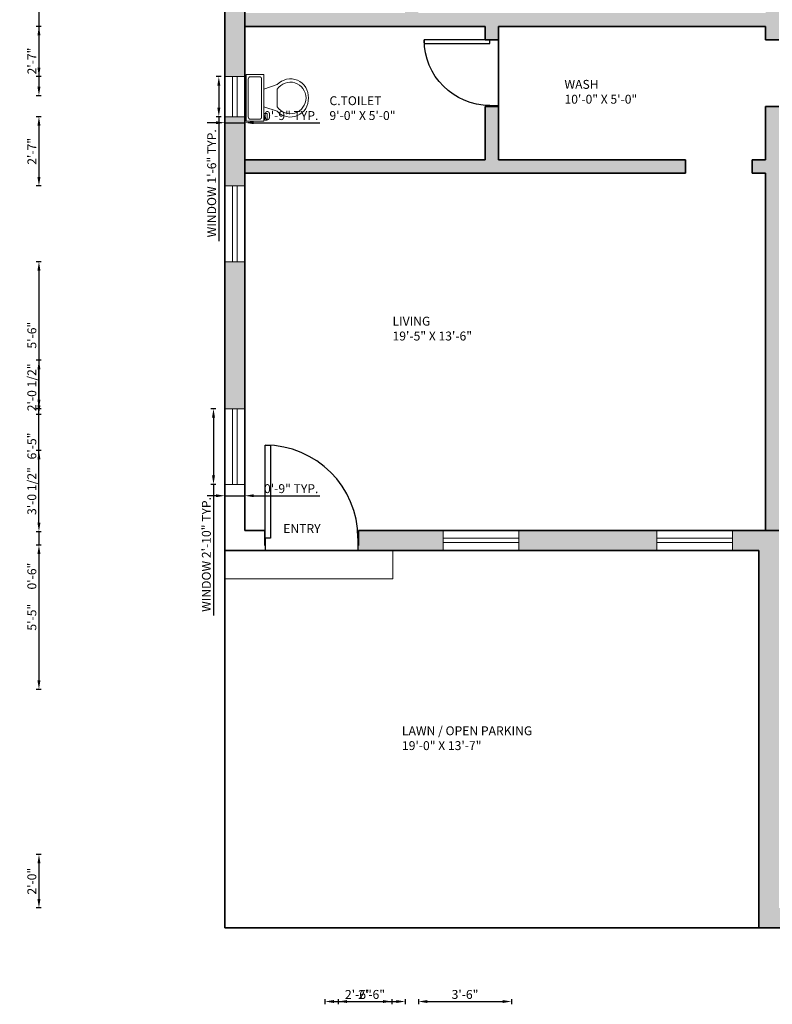
# Model space of a CAD drawing. Units: inches. Extents: x -91 to 518, y -600 to 105.
# Tile 1 of 4: x -91 to 248, y -598 to -155. Entities that reach past the tile are written whole.
import ezdxf

# ---------------------------------------------------------------- set-up
doc = ezdxf.new("R2010")
doc.units = ezdxf.units.IN
for name, color, linetype, lineweight in [('A-ANNO-DIMS', 2, 'Continuous', 18), ('A-ANNO-TEXT', 7, 'Continuous', 18), ('A-AREA-IDEN', 7, 'Continuous', 18), ('A-DOOR', 4, 'Continuous', 25), ('A-FLOR-FIXT', 9, 'Continuous', 18), ('A-FLOR-STRS', 7, 'Continuous', 18), ('A-GLAZ', 6, 'Continuous', 18), ('A-WALL', 7, 'Continuous', 35), ('A-WALL-PATT', 251, 'Continuous', 13)]:
    doc.layers.add(name, color=color, linetype=linetype, lineweight=lineweight)
doc.styles.get("Standard").update_dxf_attribs({"font": 'arial.ttf'})
doc.dimstyles.new('ISO-25', dxfattribs={"dimtxt": 4, "dimasz": 4, "dimexe": 1.25, "dimexo": 0.625, "dimtad": 1, "dimlunit": 3, "dimtxsty": 'Standard', "dimcen": 2.5, "dimadec": 0, "dimazin": 0, "dimtfac": 1, "dimtmove": 0, "dimatfit": 3, "dimfxl": 1, "dimfxlon": 1, "dimarcsym": 0})

# ---------------------------------------------------------------- blocks, each defined once
blk = doc.blocks.new('*U4')
for p, q in [((9.5, -6), (9.5, -2)), ((-10, -8.5), (-8, -8.5)), ((-10, -9.5), (-10, -8.5)), ((-8, -8.5), (-8, -8)), ((-7, -8), (-7, -9.5)), ((-4, -8), (-6, -14)), ((4, -8), (6, -14)), ((-7, -9.5), (-10, -9.5)), ((4, -14), (-4, -14))]:
    blk.add_line(p, q)
blk.add_lwpolyline([(10.5, -8), (10.5, 0), (-10.5, 0), (-10.5, -8)], close=True)
for points in [[(-9.5, -2), (-9.5, -6)], [(8.5, -1), (-8.5, -1)], [(-8.5, -7), (8.5, -7)]]:
    blk.add_lwpolyline(points)
for centre, radius, start, end in [((-8.625, -1.875), 0.8839, 81.8699, 188.1301), ((8.625, -1.875), 0.8839, 351.8699, 98.1301), ((-8.625, -6.125), 0.8839, 171.869898, 278.1301), ((8.625, -6.125), 0.8839, 261.8699, 8.1301), ((-0.4772, -19.9188), 8.0953, 133.01722, 273.38), ((0.0374, -19.8731), 7.127, 124.50543, 269.7), ((-0.0373, -19.8731), 7.127, 270.3, 55.4946), ((0.4773, -19.9188), 8.0953, 266.62, 46.9828)]:
    blk.add_arc(centre, radius, start, end)
blk = doc.blocks.new('*U2')
for p, q in [((0, 0), (0, -100)), ((750, 0), (750, -100))]:
    blk.add_line(p, q)
blk.add_lwpolyline([(0, 0), (0, 750), (43.75, 750), (43.75, 0)], close=True)
blk.add_arc((0, 0), 750, 0, 90)
blk = doc.blocks.new('WIN-34IN')
for p, q in [((0, 5.5), (34, 5.5)), ((0, 3.5), (34, 3.5))]:
    blk.add_line(p, q)
blk.add_lwpolyline([(0, 9), (34, 9), (34, 0), (0, 0)], close=True)
blk = doc.blocks.new('WIN-18IN')
for p, q in [((0, 5.5), (18, 5.5)), ((0, 3.5), (18, 3.5))]:
    blk.add_line(p, q)
blk.add_lwpolyline([(0, 9), (18, 9), (18, 0), (0, 0)], close=True)
blk = doc.blocks.new('*D18')
at = {"layer": 'A-ANNO-DIMS', "color": 0, "lineweight": -2, "transparency": 16777216}
for p, q in [((-2.56, -330.05), (-4.81, -330.05)), ((-3.56, -334.05), (-3.56, -360.05)), ((-2.56, -364.05), (-4.81, -364.05)), ((-3.56, -364.05), (-3.56, -423.02))]:
    blk.add_line(p, q, dxfattribs=at)
at = {"layer": 'A-ANNO-DIMS', "color": 0, "transparency": 16777216}
for points in [[(-4.22, -334.05), (-2.89, -334.05), (-3.56, -330.05)], [(-4.22, -360.05), (-2.89, -360.05), (-3.56, -364.05)]]:
    blk.add_solid(points, dxfattribs=at)
at = {"layer": 'Defpoints', "color": 0, "transparency": 16777216}
for p in [(1.54, -330.05), (-3.56, -364.05), (1.54, -364.05)]:
    blk.add_point(p, dxfattribs=at)
at = {"layer": 'A-ANNO-DIMS', "color": 0, "transparency": 16777216, "insert": (-6.25, -395.53), "char_height": 4, "attachment_point": 5, "rotation": 90}
blk.add_mtext('WINDOW 2\'-10" TYP.', dxfattribs=at)
blk = doc.blocks.new('*D19')
at = {"layer": 'A-ANNO-DIMS', "color": 0, "lineweight": -2, "transparency": 16777216}
for p, q in [((-2.46, -369.15), (-6.46, -369.15)), ((1.54, -368.15), (1.54, -370.4)), ((1.54, -369.15), (10.54, -369.15)), ((10.54, -368.15), (10.54, -370.4)), ((14.54, -369.15), (44.18, -369.15))]:
    blk.add_line(p, q, dxfattribs=at)
at = {"layer": 'A-ANNO-DIMS', "color": 0, "transparency": 16777216}
for points in [[(-2.46, -368.48), (-2.46, -369.81), (1.54, -369.15)], [(14.54, -368.48), (14.54, -369.81), (10.54, -369.15)]]:
    blk.add_solid(points, dxfattribs=at)
at = {"layer": 'Defpoints', "color": 0, "transparency": 16777216}
for p in [(1.54, -364.05), (10.54, -364.05), (10.54, -369.15)]:
    blk.add_point(p, dxfattribs=at)
at = {"layer": 'A-ANNO-DIMS', "color": 0, "transparency": 16777216, "insert": (31.36, -366.48), "char_height": 4, "attachment_point": 5}
blk.add_mtext('0\'-9" TYP.', dxfattribs=at)
blk = doc.blocks.new('*D20')
at = {"layer": 'A-ANNO-DIMS', "color": 0, "lineweight": -2, "transparency": 16777216}
for p, q in [((-0.16, -180.88), (-2.41, -180.88)), ((-1.16, -184.88), (-1.16, -194.88)), ((-0.16, -198.88), (-2.41, -198.88)), ((-1.16, -198.88), (-1.16, -254.74))]:
    blk.add_line(p, q, dxfattribs=at)
at = {"layer": 'A-ANNO-DIMS', "color": 0, "transparency": 16777216}
for points in [[(-1.82, -184.88), (-0.49, -184.88), (-1.16, -180.88)], [(-1.82, -194.88), (-0.49, -194.88), (-1.16, -198.88)]]:
    blk.add_solid(points, dxfattribs=at)
at = {"layer": 'Defpoints', "color": 0, "transparency": 16777216}
for p in [(1.54, -180.88), (-1.16, -198.88), (1.54, -198.88)]:
    blk.add_point(p, dxfattribs=at)
at = {"layer": 'A-ANNO-DIMS', "color": 0, "transparency": 16777216, "insert": (-3.85, -228.81), "char_height": 4, "attachment_point": 5, "rotation": 90}
blk.add_mtext('WINDOW 1\'-6" TYP.', dxfattribs=at)
blk = doc.blocks.new('*D21')
at = {"layer": 'A-ANNO-DIMS', "color": 0, "lineweight": -2, "transparency": 16777216}
for p, q in [((-2.46, -201.58), (-6.46, -201.58)), ((1.54, -200.58), (1.54, -202.83)), ((1.54, -201.58), (10.54, -201.58)), ((10.54, -200.58), (10.54, -202.83)), ((14.54, -201.58), (44.18, -201.58))]:
    blk.add_line(p, q, dxfattribs=at)
at = {"layer": 'A-ANNO-DIMS', "color": 0, "transparency": 16777216}
for points in [[(-2.46, -200.91), (-2.46, -202.24), (1.54, -201.58)], [(14.54, -200.91), (14.54, -202.24), (10.54, -201.58)]]:
    blk.add_solid(points, dxfattribs=at)
at = {"layer": 'Defpoints', "color": 0, "transparency": 16777216}
for p in [(1.54, -198.88), (10.54, -198.88), (10.54, -201.58)]:
    blk.add_point(p, dxfattribs=at)
at = {"layer": 'A-ANNO-DIMS', "color": 0, "transparency": 16777216, "insert": (31.36, -198.91), "char_height": 4, "attachment_point": 5}
blk.add_mtext('0\'-9" TYP.', dxfattribs=at)
blk = doc.blocks.new('*D32')
at = {"layer": 'A-ANNO-DIMS', "color": 0, "lineweight": -2, "transparency": 16777216}
for p, q in [((19.54, 95.59), (19.54, 97.84)), ((61.54, 95.59), (61.54, 97.84)), ((23.54, 96.59), (57.54, 96.59))]:
    blk.add_line(p, q, dxfattribs=at)
at = {"layer": 'A-ANNO-DIMS', "color": 0, "transparency": 16777216}
for points in [[(23.54, 97.25), (23.54, 95.92), (19.54, 96.59)], [(57.54, 97.25), (57.54, 95.92), (61.54, 96.59)]]:
    blk.add_solid(points, dxfattribs=at)
at = {"layer": 'Defpoints', "color": 0, "transparency": 16777216}
for p in [(61.54, 96.59), (19.54, -384.72), (61.54, -384.72)]:
    blk.add_point(p, dxfattribs=at)
at = {"layer": 'A-ANNO-DIMS', "color": 0, "transparency": 16777216, "insert": (40.54, 99.26), "char_height": 4, "attachment_point": 5}
blk.add_mtext('3\'-6"', dxfattribs=at)
blk = doc.blocks.new('*D34')
at = {"layer": 'A-ANNO-DIMS', "color": 0, "lineweight": -2, "transparency": 16777216}
for p, q in [((46.54, -595.36), (46.54, -597.61)), ((50.54, -596.36), (72.54, -596.36)), ((76.54, -595.36), (76.54, -597.61))]:
    blk.add_line(p, q, dxfattribs=at)
at = {"layer": 'A-ANNO-DIMS', "color": 0, "transparency": 16777216}
for points in [[(50.54, -595.69), (50.54, -597.02), (46.54, -596.36)], [(72.54, -595.69), (72.54, -597.02), (76.54, -596.36)]]:
    blk.add_solid(points, dxfattribs=at)
at = {"layer": 'Defpoints', "color": 0, "transparency": 16777216}
for p in [(46.54, -98.31), (76.54, -98.31), (76.54, -596.36)]:
    blk.add_point(p, dxfattribs=at)
at = {"layer": 'A-ANNO-DIMS', "color": 0, "transparency": 16777216, "insert": (61.54, -593.69), "char_height": 4, "attachment_point": 5}
blk.add_mtext('2\'-6"', dxfattribs=at)
blk = doc.blocks.new('*D35')
at = {"layer": 'A-ANNO-DIMS', "color": 0, "lineweight": -2, "transparency": 16777216}
for p, q in [((-81.99, -381.31), (-81.99, -377.31)), ((-80.99, -385.31), (-83.24, -385.31)), ((-81.99, -385.31), (-81.99, -391.31)), ((-80.99, -391.31), (-83.24, -391.31)), ((-81.99, -395.31), (-81.99, -411.19))]:
    blk.add_line(p, q, dxfattribs=at)
at = {"layer": 'A-ANNO-DIMS', "color": 0, "transparency": 16777216}
for points in [[(-82.66, -381.31), (-81.32, -381.31), (-81.99, -385.31)], [(-82.66, -395.31), (-81.32, -395.31), (-81.99, -391.31)]]:
    blk.add_solid(points, dxfattribs=at)
at = {"layer": 'Defpoints', "color": 0, "transparency": 16777216}
for p in [(310.54, -385.31), (-81.99, -391.31), (310.54, -391.31)]:
    blk.add_point(p, dxfattribs=at)
at = {"layer": 'A-ANNO-DIMS', "color": 0, "transparency": 16777216, "insert": (-84.66, -405.25), "char_height": 4, "attachment_point": 5, "rotation": 90}
blk.add_mtext('0\'-6"', dxfattribs=at)
blk = doc.blocks.new('*D36')
at = {"layer": 'A-ANNO-DIMS', "color": 0, "lineweight": -2, "transparency": 16777216}
for p, q in [((-80.99, -308.31), (-83.24, -308.31)), ((-81.99, -381.31), (-81.99, -312.31)), ((-80.99, -385.31), (-83.24, -385.31))]:
    blk.add_line(p, q, dxfattribs=at)
at = {"layer": 'A-ANNO-DIMS', "color": 0, "transparency": 16777216}
for points in [[(-82.66, -312.31), (-81.32, -312.31), (-81.99, -308.31)], [(-82.66, -381.31), (-81.32, -381.31), (-81.99, -385.31)]]:
    blk.add_solid(points, dxfattribs=at)
at = {"layer": 'Defpoints', "color": 0, "transparency": 16777216}
for p in [(-81.99, -308.31), (472.54, -308.31), (472.54, -385.31)]:
    blk.add_point(p, dxfattribs=at)
at = {"layer": 'A-ANNO-DIMS', "color": 0, "transparency": 16777216, "insert": (-84.66, -346.81), "char_height": 4, "attachment_point": 5, "rotation": 90}
blk.add_mtext('6\'-5"', dxfattribs=at)
blk = doc.blocks.new('*D37')
at = {"layer": 'A-ANNO-DIMS', "color": 0, "lineweight": -2, "transparency": 16777216}
for p, q in [((-80.99, -530.31), (-83.24, -530.31)), ((-81.99, -534.31), (-81.99, -550.31)), ((-80.99, -554.31), (-83.24, -554.31))]:
    blk.add_line(p, q, dxfattribs=at)
at = {"layer": 'A-ANNO-DIMS', "color": 0, "transparency": 16777216}
for points in [[(-82.66, -534.31), (-81.32, -534.31), (-81.99, -530.31)], [(-82.66, -550.31), (-81.32, -550.31), (-81.99, -554.31)]]:
    blk.add_solid(points, dxfattribs=at)
at = {"layer": 'Defpoints', "color": 0, "transparency": 16777216}
for p in [(375.09, -530.31), (-81.99, -554.31), (375.09, -554.31)]:
    blk.add_point(p, dxfattribs=at)
at = {"layer": 'A-ANNO-DIMS', "color": 0, "transparency": 16777216, "insert": (-84.66, -542.31), "char_height": 4, "attachment_point": 5, "rotation": 90}
blk.add_mtext('2\'-0"', dxfattribs=at)
blk = doc.blocks.new('*D41')
at = {"layer": 'A-ANNO-DIMS', "color": 0, "lineweight": -2, "transparency": 16777216}
for p, q in [((-80.99, 12.69), (-83.24, 12.69)), ((-81.99, 8.69), (-81.99, -176.88)), ((-80.99, -180.88), (-83.24, -180.88))]:
    blk.add_line(p, q, dxfattribs=at)
at = {"layer": 'A-ANNO-DIMS', "color": 0, "transparency": 16777216}
for points in [[(-82.66, 8.69), (-81.32, 8.69), (-81.99, 12.69)], [(-82.66, -176.88), (-81.32, -176.88), (-81.99, -180.88)]]:
    blk.add_solid(points, dxfattribs=at)
at = {"layer": 'Defpoints', "color": 0, "transparency": 16777216}
for p in [(1.54, 12.69), (-81.99, -180.88), (1.54, -180.88)]:
    blk.add_point(p, dxfattribs=at)
at = {"layer": 'A-ANNO-DIMS', "color": 0, "transparency": 16777216, "insert": (-84.68, -84.09), "char_height": 4, "attachment_point": 5, "rotation": 90}
blk.add_mtext('16\'-1 1/2"', dxfattribs=at)
blk = doc.blocks.new('*D42')
at = {"layer": 'A-ANNO-DIMS', "color": 0, "lineweight": -2, "transparency": 16777216}
for p, q in [((-80.99, -198.88), (-83.24, -198.88)), ((-81.99, -202.88), (-81.99, -226.01)), ((-80.99, -230.01), (-83.24, -230.01))]:
    blk.add_line(p, q, dxfattribs=at)
at = {"layer": 'A-ANNO-DIMS', "color": 0, "transparency": 16777216}
for points in [[(-82.66, -202.88), (-81.32, -202.88), (-81.99, -198.88)], [(-82.66, -226.01), (-81.32, -226.01), (-81.99, -230.01)]]:
    blk.add_solid(points, dxfattribs=at)
at = {"layer": 'Defpoints', "color": 0, "transparency": 16777216}
for p in [(1.54, -198.88), (-81.99, -230.01), (1.54, -230.01)]:
    blk.add_point(p, dxfattribs=at)
at = {"layer": 'A-ANNO-DIMS', "color": 0, "transparency": 16777216, "insert": (-84.62, -214.45), "char_height": 4, "attachment_point": 5, "rotation": 90}
blk.add_mtext('2\'-7"', dxfattribs=at)
blk = doc.blocks.new('*D43')
at = {"layer": 'A-ANNO-DIMS', "color": 0, "lineweight": -2, "transparency": 16777216}
for p, q in [((-80.99, -264.01), (-83.24, -264.01)), ((-81.99, -268.01), (-81.99, -326.05)), ((-80.99, -330.05), (-83.24, -330.05))]:
    blk.add_line(p, q, dxfattribs=at)
at = {"layer": 'A-ANNO-DIMS', "color": 0, "transparency": 16777216}
for points in [[(-82.66, -268.01), (-81.32, -268.01), (-81.99, -264.01)], [(-82.66, -326.05), (-81.32, -326.05), (-81.99, -330.05)]]:
    blk.add_solid(points, dxfattribs=at)
at = {"layer": 'Defpoints', "color": 0, "transparency": 16777216}
for p in [(1.54, -264.01), (-81.99, -330.05), (1.54, -330.05)]:
    blk.add_point(p, dxfattribs=at)
at = {"layer": 'A-ANNO-DIMS', "color": 0, "transparency": 16777216, "insert": (-84.66, -297.03), "char_height": 4, "attachment_point": 5, "rotation": 90}
blk.add_mtext('5\'-6"', dxfattribs=at)
blk = doc.blocks.new('*D44')
at = {"layer": 'A-ANNO-DIMS', "color": 0, "lineweight": -2, "transparency": 16777216}
for p, q in [((52.46, -595.36), (52.46, -597.61)), ((56.46, -596.36), (78.54, -596.36)), ((82.54, -595.36), (82.54, -597.61))]:
    blk.add_line(p, q, dxfattribs=at)
at = {"layer": 'A-ANNO-DIMS', "color": 0, "transparency": 16777216}
for points in [[(56.46, -595.69), (56.46, -597.02), (52.46, -596.36)], [(78.54, -595.69), (78.54, -597.02), (82.54, -596.36)]]:
    blk.add_solid(points, dxfattribs=at)
at = {"layer": 'Defpoints', "color": 0, "transparency": 16777216}
for p in [(52.46, 3.69), (82.54, 3.69), (82.54, -596.36)]:
    blk.add_point(p, dxfattribs=at)
at = {"layer": 'A-ANNO-DIMS', "color": 0, "transparency": 16777216, "insert": (67.5, -593.69), "char_height": 4, "attachment_point": 5}
blk.add_mtext('2\'-6"', dxfattribs=at)
blk = doc.blocks.new('*D45')
at = {"layer": 'A-ANNO-DIMS', "color": 0, "lineweight": -2, "transparency": 16777216}
for p, q in [((88.54, -595.36), (88.54, -597.61)), ((92.54, -596.36), (126.38, -596.36)), ((130.38, -595.36), (130.38, -597.61))]:
    blk.add_line(p, q, dxfattribs=at)
at = {"layer": 'A-ANNO-DIMS', "color": 0, "transparency": 16777216}
for points in [[(92.54, -595.69), (92.54, -597.02), (88.54, -596.36)], [(126.38, -595.69), (126.38, -597.02), (130.38, -596.36)]]:
    blk.add_solid(points, dxfattribs=at)
at = {"layer": 'Defpoints', "color": 0, "transparency": 16777216}
for p in [(88.54, 3.69), (130.38, 3.69), (130.38, -596.36)]:
    blk.add_point(p, dxfattribs=at)
at = {"layer": 'A-ANNO-DIMS', "color": 0, "transparency": 16777216, "insert": (109.46, -593.69), "char_height": 4, "attachment_point": 5}
blk.add_mtext('3\'-6"', dxfattribs=at)
blk = doc.blocks.new('*D48')
at = {"layer": 'A-ANNO-DIMS', "color": 0, "lineweight": -2, "transparency": 16777216}
for p, q in [((-80.99, -158.31), (-83.24, -158.31)), ((-81.99, -162.31), (-81.99, -185.45)), ((-80.99, -189.45), (-83.24, -189.45))]:
    blk.add_line(p, q, dxfattribs=at)
at = {"layer": 'A-ANNO-DIMS', "color": 0, "transparency": 16777216}
for points in [[(-82.66, -162.31), (-81.32, -162.31), (-81.99, -158.31)], [(-82.66, -185.45), (-81.32, -185.45), (-81.99, -189.45)]]:
    blk.add_solid(points, dxfattribs=at)
at = {"layer": 'Defpoints', "color": 0, "transparency": 16777216}
for p in [(472.54, -158.31), (-81.99, -189.45), (472.54, -189.45)]:
    blk.add_point(p, dxfattribs=at)
at = {"layer": 'A-ANNO-DIMS', "color": 0, "transparency": 16777216, "insert": (-84.62, -173.88), "char_height": 4, "attachment_point": 5, "rotation": 90}
blk.add_mtext('2\'-7"', dxfattribs=at)
blk = doc.blocks.new('*D49')
at = {"layer": 'A-ANNO-DIMS', "color": 0, "lineweight": -2, "transparency": 16777216}
for p, q in [((-80.99, -308.31), (-83.24, -308.31)), ((-81.99, -312.31), (-81.99, -328.59)), ((-80.99, -332.59), (-83.24, -332.59))]:
    blk.add_line(p, q, dxfattribs=at)
at = {"layer": 'A-ANNO-DIMS', "color": 0, "transparency": 16777216}
for points in [[(-82.66, -312.31), (-81.32, -312.31), (-81.99, -308.31)], [(-82.66, -328.59), (-81.32, -328.59), (-81.99, -332.59)]]:
    blk.add_solid(points, dxfattribs=at)
at = {"layer": 'Defpoints', "color": 0, "transparency": 16777216}
for p in [(472.54, -308.31), (-81.99, -332.59), (472.54, -332.59)]:
    blk.add_point(p, dxfattribs=at)
at = {"layer": 'A-ANNO-DIMS', "color": 0, "transparency": 16777216, "insert": (-84.68, -320.45), "char_height": 4, "attachment_point": 5, "rotation": 90}
blk.add_mtext('2\'-0 1/2"', dxfattribs=at)
blk = doc.blocks.new('*D50')
at = {"layer": 'A-ANNO-DIMS', "color": 0, "lineweight": -2, "transparency": 16777216}
for p, q in [((-80.99, -391.31), (-83.24, -391.31)), ((-81.99, -395.31), (-81.99, -452.14)), ((-80.99, -456.14), (-83.24, -456.14))]:
    blk.add_line(p, q, dxfattribs=at)
at = {"layer": 'A-ANNO-DIMS', "color": 0, "transparency": 16777216}
for points in [[(-82.66, -395.31), (-81.32, -395.31), (-81.99, -391.31)], [(-82.66, -452.14), (-81.32, -452.14), (-81.99, -456.14)]]:
    blk.add_solid(points, dxfattribs=at)
at = {"layer": 'Defpoints', "color": 0, "transparency": 16777216}
for p in [(472.54, -391.31), (-81.99, -456.14), (472.54, -456.14)]:
    blk.add_point(p, dxfattribs=at)
at = {"layer": 'A-ANNO-DIMS', "color": 0, "transparency": 16777216, "insert": (-84.65, -423.72), "char_height": 4, "attachment_point": 5, "rotation": 90}
blk.add_mtext('5\'-5"', dxfattribs=at)
blk = doc.blocks.new('*D52')
at = {"layer": 'A-ANNO-DIMS', "color": 0, "lineweight": -2, "transparency": 16777216}
for p, q in [((61.33, 95.59), (61.33, 97.84)), ((99.7, 95.59), (99.7, 97.84)), ((65.33, 96.59), (95.7, 96.59))]:
    blk.add_line(p, q, dxfattribs=at)
at = {"layer": 'A-ANNO-DIMS', "color": 0, "transparency": 16777216}
for points in [[(65.33, 97.25), (65.33, 95.92), (61.33, 96.59)], [(95.7, 97.25), (95.7, 95.92), (99.7, 96.59)]]:
    blk.add_solid(points, dxfattribs=at)
at = {"layer": 'Defpoints', "color": 0, "transparency": 16777216}
for p in [(99.7, 96.59), (61.33, -393.72), (99.7, -393.72)]:
    blk.add_point(p, dxfattribs=at)
at = {"layer": 'A-ANNO-DIMS', "color": 0, "transparency": 16777216, "insert": (80.52, 99.28), "char_height": 4, "attachment_point": 5}
blk.add_mtext('3\'-2 1/2"', dxfattribs=at)
blk = doc.blocks.new('*D53')
at = {"layer": 'A-ANNO-DIMS', "color": 0, "lineweight": -2, "transparency": 16777216}
for p, q in [((133.7, 95.59), (133.7, 97.84)), ((195.65, 95.59), (195.65, 97.84)), ((137.7, 96.59), (191.65, 96.59))]:
    blk.add_line(p, q, dxfattribs=at)
at = {"layer": 'A-ANNO-DIMS', "color": 0, "transparency": 16777216}
for points in [[(137.7, 97.25), (137.7, 95.92), (133.7, 96.59)], [(191.65, 97.25), (191.65, 95.92), (195.65, 96.59)]]:
    blk.add_solid(points, dxfattribs=at)
at = {"layer": 'Defpoints', "color": 0, "transparency": 16777216}
for p in [(195.65, 96.59), (133.7, -393.72), (195.65, -393.72)]:
    blk.add_point(p, dxfattribs=at)
at = {"layer": 'A-ANNO-DIMS', "color": 0, "transparency": 16777216, "insert": (164.67, 99.25), "char_height": 4, "attachment_point": 5}
blk.add_mtext('5\'-2"', dxfattribs=at)
blk = doc.blocks.new('*D56')
at = {"layer": 'A-ANNO-DIMS', "color": 0, "lineweight": -2, "transparency": 16777216}
for p, q in [((229.65, 95.59), (229.65, 97.84)), ((244.54, 95.59), (244.54, 97.84)), ((233.65, 96.59), (240.54, 96.59))]:
    blk.add_line(p, q, dxfattribs=at)
at = {"layer": 'A-ANNO-DIMS', "color": 0, "transparency": 16777216}
for points in [[(233.65, 97.25), (233.65, 95.92), (229.65, 96.59)], [(240.54, 97.25), (240.54, 95.92), (244.54, 96.59)]]:
    blk.add_solid(points, dxfattribs=at)
at = {"layer": 'Defpoints', "color": 0, "transparency": 16777216}
for p in [(244.54, 96.59), (229.65, -384.72), (244.54, -384.72)]:
    blk.add_point(p, dxfattribs=at)
at = {"layer": 'A-ANNO-DIMS', "color": 0, "transparency": 16777216, "insert": (237.09, 99.26), "char_height": 4, "attachment_point": 5}
blk.add_mtext('1\'-3"', dxfattribs=at)
blk = doc.blocks.new('*D57')
at = {"layer": 'A-ANNO-DIMS', "color": 0, "lineweight": -2, "transparency": 16777216}
for p, q in [((-80.99, -348.81), (-83.24, -348.81)), ((-81.99, -381.31), (-81.99, -352.81)), ((-80.99, -385.31), (-83.24, -385.31))]:
    blk.add_line(p, q, dxfattribs=at)
at = {"layer": 'A-ANNO-DIMS', "color": 0, "transparency": 16777216}
for points in [[(-82.66, -352.81), (-81.32, -352.81), (-81.99, -348.81)], [(-82.66, -381.31), (-81.32, -381.31), (-81.99, -385.31)]]:
    blk.add_solid(points, dxfattribs=at)
at = {"layer": 'Defpoints', "color": 0, "transparency": 16777216}
for p in [(-81.99, -348.81), (333.53, -348.81), (333.53, -385.31)]:
    blk.add_point(p, dxfattribs=at)
at = {"layer": 'A-ANNO-DIMS', "color": 0, "transparency": 16777216, "insert": (-84.68, -367.06), "char_height": 4, "attachment_point": 5, "rotation": 90}
blk.add_mtext('3\'-0 1/2"', dxfattribs=at)

msp = doc.modelspace()

# ---------------------------------------------------------------- hatches: boundary and pattern name
at = {"layer": 'A-WALL-PATT'}
h = msp.add_hatch(color=256, dxfattribs=at)
h.dxf.hatch_style = 1
h.paths.add_polyline_path([(10.544, 3.693), (34.462, 3.693), (34.462, 12.693), (1.544, 12.693), (1.544, -180.878), (10.544, -180.878)])
h.paths.add_polyline_path([(46.544, -92.307), (10.544, -92.307), (10.544, -98.307), (46.544, -98.307)])
h.paths.add_polyline_path([(130.381, 12.693), (52.462, 12.693), (52.462, 3.693), (82.544, 3.693), (88.544, 3.693), (130.381, 3.693)])
h.paths.add_polyline_path([(88.544, 3.693), (82.544, 3.693), (82.544, -92.307), (76.544, -92.307), (76.544, -94.37), (76.544, -98.307), (82.544, -98.307), (82.544, -106.057), (85.522, -106.057), (88.544, -106.057)])
h.paths.add_polyline_path([(250.544, -146.307), (245.772, -146.307), (244.544, -146.307), (244.544, -152.307), (88.544, -152.307), (88.544, -141.744), (85.718, -141.744), (82.544, -141.744), (82.544, -152.307), (10.544, -152.307), (10.544, -158.307), (88.544, -158.307), (118.544, -158.307), (118.544, -164.307), (120.607, -164.307), (124.544, -164.307), (124.544, -158.307), (244.544, -158.307), (244.544, -164.307), (250.544, -164.307)])
h.paths.add_polyline_path([(274.341, 12.693), (184.381, 12.693), (184.381, 3.693), (244.544, 3.693), (250.544, 3.693), (274.341, 3.693)])
h.paths.add_polyline_path([(250.544, 3.693), (244.544, 3.693), (244.544, -110.307), (250.544, -110.307), (250.544, -98.307), (310.544, -98.307), (310.544, -110.307), (316.544, -110.307), (316.544, -86.517), (312.607, -86.517), (310.544, -86.517), (310.544, -92.307), (250.544, -92.307)])
h.paths.add_polyline_path([(481.544, 12.693), (292.341, 12.693), (292.341, 3.693), (310.544, 3.693), (316.544, 3.693), (472.544, 3.693), (472.544, -34.129), (481.544, -34.129)])
h.paths.add_polyline_path([(316.544, 3.693), (310.544, 3.693), (310.544, -56.517), (316.544, -56.517)], flags=17)
h.paths.add_polyline_path([(481.544, -88.129), (472.544, -88.129), (472.544, -189.451), (481.544, -189.451)])
h.paths.add_polyline_path([(472.544, -152.307), (316.544, -152.307), (316.544, -146.307), (315.319, -146.307), (310.544, -146.307), (310.544, -260.307), (316.544, -260.307), (316.544, -158.307), (472.544, -158.307)])
h.paths.add_polyline_path([(481.544, -243.451), (472.544, -243.451), (472.544, -308.307), (472.544, -332.593), (481.544, -332.593)])
h.paths.add_polyline_path([(472.544, -302.307), (316.544, -302.307), (316.544, -296.307), (315.322, -296.307), (310.544, -296.307), (310.544, -308.307), (472.544, -308.307)])
h.paths.add_polyline_path([(481.544, -366.593), (472.544, -366.593), (472.544, -385.307), (472.544, -456.136), (481.544, -456.136)])
h.paths.add_polyline_path([(472.544, -385.307), (310.544, -385.307), (310.544, -391.307), (472.544, -391.307)])
h.paths.add_polyline_path([(481.544, -510.136), (472.544, -510.136), (472.544, -554.307), (323.185, -554.307), (323.185, -563.307), (481.544, -563.307)])
h.paths.add_polyline_path([(250.544, -384.724), (229.645, -384.724), (229.645, -393.724), (241.544, -393.724), (241.544, -563.307), (269.185, -563.307), (269.185, -554.307), (250.544, -554.307)])
h.paths.add_polyline_path([(195.645, -384.724), (133.7, -384.724), (133.7, -393.724), (195.645, -393.724)])
h.paths.add_polyline_path([(99.7, -384.724), (61.544, -384.724), (61.544, -391.562), (61.335, -393.724), (77.042, -393.724), (99.7, -393.724)])
h.paths.add_polyline_path([(10.544, -264.014), (1.544, -264.014), (1.544, -330.048), (10.544, -330.048)])
h.paths.add_polyline_path([(10.544, -198.878), (1.544, -198.878), (1.544, -230.014), (10.544, -230.014)])
h.paths.add_polyline_path([(208.544, -218.307), (124.544, -218.307), (124.544, -194.307), (118.544, -194.307), (118.544, -218.307), (10.544, -218.307), (10.544, -224.307), (118.544, -224.307), (124.544, -224.307), (208.544, -224.307)])
h.paths.add_polyline_path([(250.544, -194.307), (244.544, -194.307), (244.544, -218.307), (238.544, -218.307), (238.544, -224.307), (244.544, -224.307), (244.544, -384.724), (250.544, -384.724)])

# ---------------------------------------------------------------- linework, layer by layer
at = {"layer": 'A-FLOR-STRS'}
msp.add_lwpolyline([(1.544, -393.724), (77.042, -393.724), (77.042, -406.553), (1.544, -406.553)], close=True, dxfattribs=at)
at = {"layer": 'A-WALL'}
for p, q in [((1.544, -563.307), (1.544, 12.693)), ((10.544, -384.724), (10.544, 3.693)), ((88.544, -158.307), (10.544, -158.307)), ((88.544, -158.307), (118.544, -158.307)), ((118.544, -158.307), (118.544, -164.307)), ((124.544, -158.307), (124.544, -218.307)), ((124.544, -158.307), (244.544, -158.307)), ((244.544, -164.307), (244.544, -158.307)), ((124.544, -164.307), (118.544, -164.307)), ((244.544, -164.307), (250.544, -164.307)), ((124.544, -194.307), (118.544, -194.307)), ((118.544, -194.307), (118.544, -218.307)), ((244.544, -194.307), (250.544, -194.307)), ((244.544, -218.307), (244.544, -194.307)), ((118.544, -218.307), (10.544, -218.307)), ((124.544, -218.307), (208.544, -218.307)), ((208.544, -218.307), (208.544, -224.307)), ((238.544, -218.307), (238.544, -224.307)), ((238.544, -218.307), (244.544, -218.307)), ((118.544, -224.307), (10.544, -224.307)), ((118.544, -224.307), (124.544, -224.307)), ((124.544, -224.307), (208.544, -224.307)), ((238.544, -224.307), (244.544, -224.307)), ((244.544, -224.307), (244.544, -384.724)), ((19.544, -384.724), (10.544, -384.724)), ((19.544, -384.724), (19.544, -391.562)), ((250.544, -384.724), (61.544, -384.724)), ((61.544, -384.724), (61.544, -391.562)), ((241.544, -393.724), (1.544, -393.724)), ((241.544, -393.724), (241.544, -563.307)), ((481.544, -563.307), (1.544, -563.307))]:
    msp.add_line(p, q, dxfattribs=at)

# ---------------------------------------------------------------- block references
at = {"layer": 'A-DOOR', "xscale": -0.0393700787401575, "yscale": 0.0393700787401575, "zscale": 0.0393700787401575, "rotation": 90}
msp.add_blockref('*U2', (120.607, -164.307), dxfattribs=at)
at = {"layer": 'A-DOOR', "xscale": 0.0556540566143213, "yscale": 0.0556540566143213, "zscale": 0.0556540566143213}
msp.add_blockref('*U2', (19.594, -388.158), dxfattribs=at)
at = {"layer": 'A-FLOR-FIXT', "rotation": 90}
msp.add_blockref('*U4', (11.061, -190.464), dxfattribs=at)
at = {"layer": 'A-GLAZ'}
for name, p, rotation in [('WIN-18IN', (1.544, -180.878), 270), ('WIN-34IN', (1.544, -230.014), 270.0000000000001), ('WIN-34IN', (1.544, -330.047), 270.0000000000001)]:
    msp.add_blockref(name, p, dxfattribs=dict(at, rotation=rotation))
for p in [(99.7, -393.724), (195.645, -393.724)]:
    msp.add_blockref('WIN-34IN', p, dxfattribs=at)

# ---------------------------------------------------------------- texts
at = {"layer": 'A-ANNO-TEXT', "insert": (27.784, -381.892), "char_height": 4, "attachment_point": 1}
msp.add_mtext_dynamic_manual_height_columns('ENTRY', width=20.23961, gutter_width=12.5, heights=[0], dxfattribs=at)
at = {"layer": 'A-AREA-IDEN', "char_height": 4, "attachment_point": 1}
for s, width, insert in [('WASH\\P10\'-0" X 5\'-0"', 59.48262, (154.147, -182.366)), ('C.TOILET\\P9\'-0" X 5\'-0"', 52.36634, (48.541, -189.701)), ('LIVING\\P19\'-5" X 13\'-6"', 117.96426, (76.885, -288.74)), ('LAWN / OPEN PARKING\\P19\'-0" X 13\'-7"', 149.97124, (81.117, -472.734))]:
    msp.add_mtext_dynamic_manual_height_columns(s, width=width, gutter_width=12.5, heights=[0], dxfattribs=dict(at, insert=insert))

# ---------------------------------------------------------------- dimensions: what is measured, and where the dimension line sits
at = {"layer": 'A-ANNO-DIMS'}
for base, p1, p2, picture, middle in [((61.544, 96.588), (19.544, -384.724), (61.544, -384.724), '*D32', (40.544, 99.256)), ((99.7, 96.588), (61.335, -393.724), (99.7, -393.724), '*D52', (80.518, 99.282)), ((195.645, 96.588), (133.7, -393.724), (195.645, -393.724), '*D53', (164.673, 99.255)), ((244.544, 96.588), (229.645, -384.724), (244.544, -384.724), '*D56', (237.095, 99.256)), ((82.544, -596.357), (52.462, 3.693), (82.544, 3.693), '*D44', (67.503, -593.69)), ((130.381, -596.357), (88.544, 3.693), (130.381, 3.688), '*D45', (109.462, -593.688)), ((76.544, -596.357), (46.544, -98.307), (76.544, -98.307), '*D34', (61.544, -593.69))]:
    dim = msp.add_linear_dim(base=base, p1=p1, p2=p2, dimstyle='ISO-25', override={"dimdec": 1, "dimlfac": 1, "dimrnd": 0, "dimzin": 1, "dimdsep": 46, "dimlunit": 4, "dimfrac": 2}, dxfattribs=at)
    dim.commit()
    dim.dimension.update_dxf_attribs({"geometry": picture, "text_midpoint": middle})
for base, p1, p2, picture, middle in [((-81.989, -180.878), (1.544, 12.693), (1.544, -180.878), '*D41', (-84.682, -84.092)), ((-81.989, -189.451), (472.544, -158.307), (472.544, -189.451), '*D48', (-84.622, -173.879)), ((-81.989, -230.014), (1.544, -198.878), (1.544, -230.014), '*D42', (-84.622, -214.446)), ((-81.989, -330.048), (1.544, -264.014), (1.544, -330.048), '*D43', (-84.656, -297.031)), ((-81.989, -332.593), (472.544, -308.307), (472.544, -332.593), '*D49', (-84.682, -320.45)), ((-81.989, -308.307), (472.544, -385.307), (472.544, -308.307), '*D36', (-84.656, -346.807)), ((-81.989, -348.807), (333.532, -385.307), (333.532, -348.807), '*D57', (-84.683, -367.057)), ((-81.989, -391.307), (310.544, -385.307), (310.544, -391.307), '*D35', (-84.656, -405.249)), ((-81.989, -456.136), (472.544, -391.307), (472.544, -456.136), '*D50', (-84.648, -423.722)), ((-81.989, -554.307), (375.087, -530.307), (375.087, -554.307), '*D37', (-84.656, -542.307))]:
    dim = msp.add_linear_dim(base=base, p1=p1, p2=p2, angle=90, dimstyle='ISO-25', override={"dimdec": 1, "dimlfac": 1, "dimrnd": 0, "dimzin": 1, "dimdsep": 46, "dimlunit": 4, "dimfrac": 2}, dxfattribs=at)
    dim.commit()
    dim.dimension.update_dxf_attribs({"geometry": picture, "text_midpoint": middle})
for base, p1, p2, picture, middle in [((-1.156, -198.878), (1.544, -180.878), (1.544, -198.878), '*D20', (-3.851, -228.811)), ((-3.556, -364.048), (1.544, -330.048), (1.544, -364.048), '*D18', (-6.251, -395.535))]:
    dim = msp.add_linear_dim(base=base, p1=p1, p2=p2, angle=270, text='WINDOW <> TYP.', dimstyle='ISO-25', override={"dimdec": 1, "dimlfac": 1, "dimrnd": 0, "dimzin": 1, "dimdsep": 46, "dimlunit": 4, "dimfrac": 2}, dxfattribs=at)
    dim.commit()
    dim.dimension.update_dxf_attribs({"geometry": picture, "text_midpoint": middle})
for base, p1, p2, picture, middle in [((10.544, -201.578), (1.544, -198.878), (10.544, -198.878), '*D21', (31.36, -198.91)), ((10.544, -369.148), (1.544, -364.048), (10.544, -364.048), '*D19', (31.36, -366.48))]:
    dim = msp.add_linear_dim(base=base, p1=p1, p2=p2, text='<> TYP.', dimstyle='ISO-25', override={"dimdec": 1, "dimlfac": 1, "dimrnd": 0, "dimzin": 1, "dimdsep": 46, "dimlunit": 4, "dimfrac": 2}, dxfattribs=at)
    dim.commit()
    dim.dimension.update_dxf_attribs({"geometry": picture, "text_midpoint": middle})

doc.saveas('drawing.dxf')
